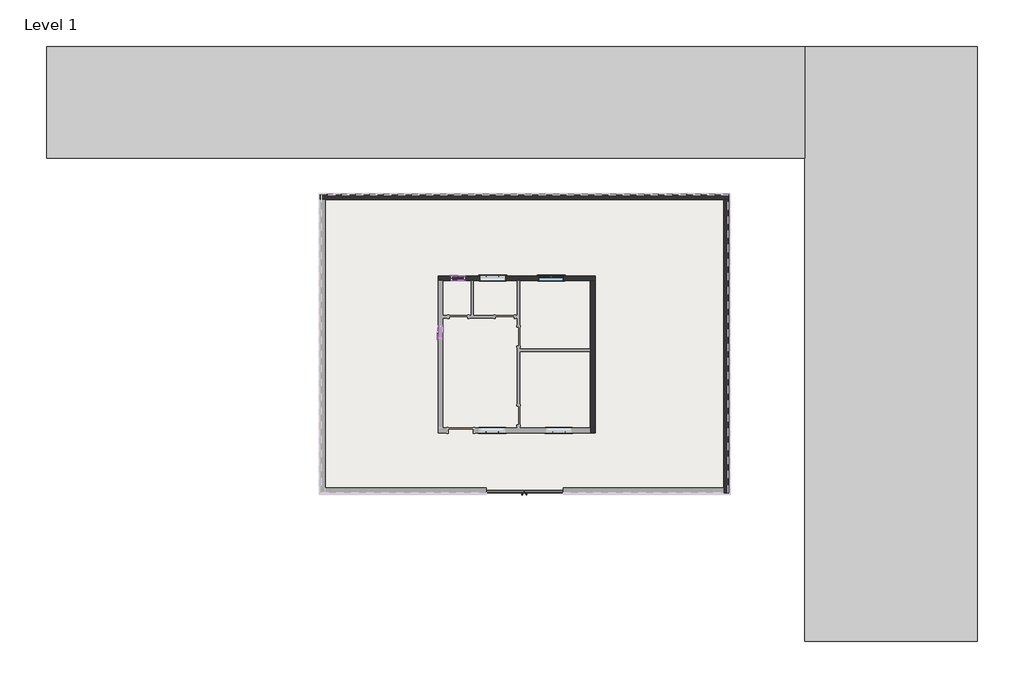
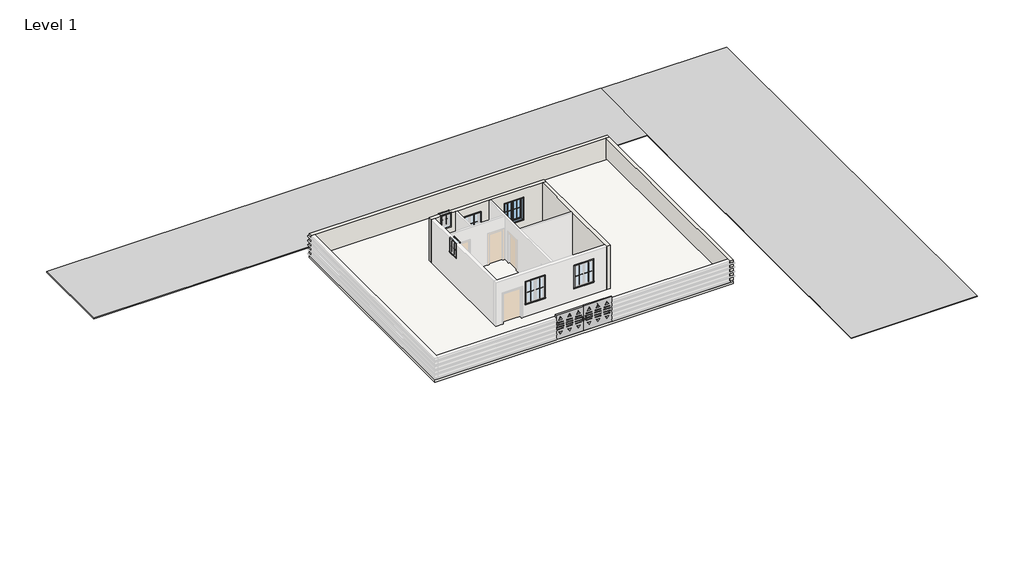
# One storey, part 2 of 2: 26 proxies, 4 walls, 1 slab, 1 window.
"""IFC4 building model written with IfcOpenShell, lengths in millimetres."""

from ifc_helpers import new_model, si_unit, frame, origin, place, context, project, spatial, polyline, outline, extrude, faceted_brep, transform, mapped, element, save
from components import generic_models_afecbd1f, generic_models_1_generic_models_1_fe68cf6e, muntin_pattern_2x2_muntin_pattern_2x2_6dad3731, muntin_pattern_2x2_muntin_pattern_2x2_a30a3345, muntin_pattern_2x2_muntin_pattern_2x2_53152e2c, muntin_pattern_2x2_muntin_pattern_2x2_e8f3e573, trim_window_exterior_flat_with_sill_92b9b949, trim_window_exterior_flat_with_sill_a665a915, trim_window_interior_flat_picture_frame_3bb882cf, trim_window_interior_flat_picture_frame_d485c387, window_8377141f

model = new_model("IFC4")

# Units and contexts
model_context = context("Model", 3, world=origin())
ifc_project = project(units=[si_unit("LENGTHUNIT", "METRE", prefix="MILLI")], contexts=[model_context])

# Site, building, storey
site = spatial("IfcSite", under=ifc_project)
building = spatial("IfcBuilding", under=site)
storey = spatial("IfcBuildingStorey", under=building, Name="Level 1", Elevation=0.0)

# Proxies
placement = place(None, origin())
generic_models_shape = generic_models_afecbd1f(model_context)
element("IfcBuildingElementProxy", 1, Name="Generic Models", at=placement, inside=storey, context=model_context, shape_type="MappedRepresentation", body=[
    mapped(generic_models_shape, transform((4902.2, 3557.455505, 0.0), x_axis=(1.0, 0.0, 0.0), y_axis=(0.0, 1.0, 0.0), z_axis=(0.0, 0.0, 1.0))),
])
generic_models_1_generic_models_1_shape = generic_models_1_generic_models_1_fe68cf6e(model_context)
element("IfcBuildingElementProxy", 2, Name="Generic Models 1 : Generic Models 1", ObjectType="Generic Models 1 : Generic Models 1", at=placement, inside=storey, context=model_context, shape_type="MappedRepresentation", body=[
    mapped(generic_models_1_generic_models_1_shape, transform((0.0, 0.0, 0.0), x_axis=(1.0, 0.0, 0.0), y_axis=(0.0, 1.0, 0.0), z_axis=(0.0, 0.0, 1.0))),
])
muntin_pattern_2x2_muntin_pattern_2x2_shape = muntin_pattern_2x2_muntin_pattern_2x2_6dad3731(model_context)
element("IfcBuildingElementProxy", 3, Name="Muntin Pattern_2x2 : Muntin Pattern_2x2", ObjectType="Muntin Pattern_2x2 : Muntin Pattern_2x2", at=placement, inside=storey, context=model_context, shape_type="MappedRepresentation", body=[
    mapped(muntin_pattern_2x2_muntin_pattern_2x2_shape, transform((6199.1875, 13960.475, 984.25), x_axis=(1.0, 0.0, 0.0), y_axis=(0.0, 1.0, 0.0), z_axis=(0.0, 0.0, 1.0))),
])
element("IfcBuildingElementProxy", 4, Name="Muntin Pattern_2x2 : Muntin Pattern_2x2", ObjectType="Muntin Pattern_2x2 : Muntin Pattern_2x2", at=placement, inside=storey, context=model_context, shape_type="MappedRepresentation", body=[
    mapped(muntin_pattern_2x2_muntin_pattern_2x2_shape, transform((7186.6125, 6359.525, 984.25), x_axis=(-1.0, 0.0, 0.0), y_axis=(0.0, -1.0, 0.0), z_axis=(0.0, 0.0, 1.0))),
])
element("IfcBuildingElementProxy", 5, Name="Muntin Pattern_2x2 : Muntin Pattern_2x2", ObjectType="Muntin Pattern_2x2 : Muntin Pattern_2x2", at=placement, inside=storey, context=model_context, shape_type="MappedRepresentation", body=[
    mapped(muntin_pattern_2x2_muntin_pattern_2x2_shape, transform((3948.1125, 6359.525, 984.25), x_axis=(-1.0, 0.0, 0.0), y_axis=(0.0, -1.0, 0.0), z_axis=(0.0, 0.0, 1.0))),
])
element("IfcBuildingElementProxy", 6, Name="Muntin Pattern_2x2 : Muntin Pattern_2x2", ObjectType="Muntin Pattern_2x2 : Muntin Pattern_2x2", at=placement, inside=storey, context=model_context, shape_type="MappedRepresentation", body=[
    mapped(muntin_pattern_2x2_muntin_pattern_2x2_shape, transform((3360.7375, 13960.475, 984.25), x_axis=(1.0, 0.0, 0.0), y_axis=(0.0, 1.0, 0.0), z_axis=(0.0, 0.0, 1.0))),
])
muntin_pattern_2x2_muntin_pattern_2x2_2_shape = muntin_pattern_2x2_muntin_pattern_2x2_a30a3345(model_context)
element("IfcBuildingElementProxy", 7, Name="Muntin Pattern_2x2 : Muntin Pattern_2x2", ObjectType="Muntin Pattern_2x2 : Muntin Pattern_2x2", at=placement, inside=storey, context=model_context, shape_type="MappedRepresentation", body=[
    mapped(muntin_pattern_2x2_muntin_pattern_2x2_2_shape, transform((6805.6125, 13960.475, 984.25), x_axis=(-1.0, 0.0, 0.0), y_axis=(0.0, -1.0, 0.0), z_axis=(0.0, 0.0, 1.0))),
])
element("IfcBuildingElementProxy", 8, Name="Muntin Pattern_2x2 : Muntin Pattern_2x2", ObjectType="Muntin Pattern_2x2 : Muntin Pattern_2x2", at=placement, inside=storey, context=model_context, shape_type="MappedRepresentation", body=[
    mapped(muntin_pattern_2x2_muntin_pattern_2x2_2_shape, transform((6580.1875, 6359.525, 984.25), x_axis=(1.0, 0.0, 0.0), y_axis=(0.0, 1.0, 0.0), z_axis=(0.0, 0.0, 1.0))),
])
element("IfcBuildingElementProxy", 9, Name="Muntin Pattern_2x2 : Muntin Pattern_2x2", ObjectType="Muntin Pattern_2x2 : Muntin Pattern_2x2", at=placement, inside=storey, context=model_context, shape_type="MappedRepresentation", body=[
    mapped(muntin_pattern_2x2_muntin_pattern_2x2_2_shape, transform((3341.6875, 6359.525, 984.25), x_axis=(1.0, 0.0, 0.0), y_axis=(0.0, 1.0, 0.0), z_axis=(0.0, 0.0, 1.0))),
])
element("IfcBuildingElementProxy", 10, Name="Muntin Pattern_2x2 : Muntin Pattern_2x2", ObjectType="Muntin Pattern_2x2 : Muntin Pattern_2x2", at=placement, inside=storey, context=model_context, shape_type="MappedRepresentation", body=[
    mapped(muntin_pattern_2x2_muntin_pattern_2x2_2_shape, transform((3967.1625, 13960.475, 984.25), x_axis=(-1.0, 0.0, 0.0), y_axis=(0.0, -1.0, 0.0), z_axis=(0.0, 0.0, 1.0))),
])
muntin_pattern_2x2_muntin_pattern_2x2_3_shape = muntin_pattern_2x2_muntin_pattern_2x2_53152e2c(model_context)
element("IfcBuildingElementProxy", 11, Name="Muntin Pattern_2x2 : Muntin Pattern_2x2", ObjectType="Muntin Pattern_2x2 : Muntin Pattern_2x2", at=placement, inside=storey, context=model_context, shape_type="MappedRepresentation", body=[
    mapped(muntin_pattern_2x2_muntin_pattern_2x2_3_shape, transform((1025.525, 11069.6375, 2203.45), x_axis=(0.0, 1.0, 0.0), y_axis=(-1.0, 0.0, 0.0), z_axis=(0.0, 0.0, 1.0))),
])
element("IfcBuildingElementProxy", 12, Name="Muntin Pattern_2x2 : Muntin Pattern_2x2", ObjectType="Muntin Pattern_2x2 : Muntin Pattern_2x2", at=placement, inside=storey, context=model_context, shape_type="MappedRepresentation", body=[
    mapped(muntin_pattern_2x2_muntin_pattern_2x2_3_shape, transform((1830.3875, 13960.475, 2203.45), x_axis=(1.0, 0.0, 0.0), y_axis=(0.0, 1.0, 0.0), z_axis=(0.0, 0.0, 1.0))),
])
muntin_pattern_2x2_muntin_pattern_2x2_4_shape = muntin_pattern_2x2_muntin_pattern_2x2_e8f3e573(model_context)
element("IfcBuildingElementProxy", 13, Name="Muntin Pattern_2x2 : Muntin Pattern_2x2", ObjectType="Muntin Pattern_2x2 : Muntin Pattern_2x2", at=placement, inside=storey, context=model_context, shape_type="MappedRepresentation", body=[
    mapped(muntin_pattern_2x2_muntin_pattern_2x2_4_shape, transform((1025.525, 11371.2625, 2203.45), x_axis=(0.0, -1.0, 0.0), y_axis=(1.0, 0.0, 0.0), z_axis=(0.0, 0.0, 1.0))),
])
element("IfcBuildingElementProxy", 14, Name="Muntin Pattern_2x2 : Muntin Pattern_2x2", ObjectType="Muntin Pattern_2x2 : Muntin Pattern_2x2", at=placement, inside=storey, context=model_context, shape_type="MappedRepresentation", body=[
    mapped(muntin_pattern_2x2_muntin_pattern_2x2_4_shape, transform((2132.0125, 13960.475, 2203.45), x_axis=(-1.0, 0.0, 0.0), y_axis=(0.0, -1.0, 0.0), z_axis=(0.0, 0.0, 1.0))),
])
trim_window_exterior_flat_with_sill_shape = trim_window_exterior_flat_with_sill_92b9b949(model_context)
element("IfcBuildingElementProxy", 15, Name="Trim-Window-Exterior-Flat : with Sill", ObjectType="Trim-Window-Exterior-Flat : with Sill", at=placement, inside=storey, context=model_context, shape_type="MappedRepresentation", body=[
    mapped(trim_window_exterior_flat_with_sill_shape, transform((6502.4, 13970.0, 2438.4), x_axis=(-1.0, 0.0, 0.0), y_axis=(0.0, 0.0, 1.0), z_axis=(0.0, 1.0, 0.0))),
])
element("IfcBuildingElementProxy", 16, Name="Trim-Window-Exterior-Flat : with Sill", ObjectType="Trim-Window-Exterior-Flat : with Sill", at=placement, inside=storey, context=model_context, shape_type="MappedRepresentation", body=[
    mapped(trim_window_exterior_flat_with_sill_shape, transform((6883.4, 6350.0, 2438.4), x_axis=(1.0, 0.0, 0.0), y_axis=(0.0, 0.0, 1.0), z_axis=(0.0, -1.0, 0.0))),
])
element("IfcBuildingElementProxy", 17, Name="Trim-Window-Exterior-Flat : with Sill", ObjectType="Trim-Window-Exterior-Flat : with Sill", at=placement, inside=storey, context=model_context, shape_type="MappedRepresentation", body=[
    mapped(trim_window_exterior_flat_with_sill_shape, transform((3644.9, 6350.0, 2438.4), x_axis=(1.0, 0.0, 0.0), y_axis=(0.0, 0.0, 1.0), z_axis=(0.0, -1.0, 0.0))),
])
element("IfcBuildingElementProxy", 18, Name="Trim-Window-Exterior-Flat : with Sill", ObjectType="Trim-Window-Exterior-Flat : with Sill", at=placement, inside=storey, context=model_context, shape_type="MappedRepresentation", body=[
    mapped(trim_window_exterior_flat_with_sill_shape, transform((3663.95, 13970.0, 2438.4), x_axis=(-1.0, 0.0, 0.0), y_axis=(0.0, 0.0, 1.0), z_axis=(0.0, 1.0, 0.0))),
])
trim_window_exterior_flat_with_sill_2_shape = trim_window_exterior_flat_with_sill_a665a915(model_context)
element("IfcBuildingElementProxy", 19, Name="Trim-Window-Exterior-Flat : with Sill", ObjectType="Trim-Window-Exterior-Flat : with Sill", at=placement, inside=storey, context=model_context, shape_type="MappedRepresentation", body=[
    mapped(trim_window_exterior_flat_with_sill_2_shape, transform((1016.0, 11220.45, 3048.0), x_axis=(0.0, -1.0, 0.0), y_axis=(0.0, 0.0, 1.0), z_axis=(-1.0, 0.0, 0.0))),
])
element("IfcBuildingElementProxy", 20, Name="Trim-Window-Exterior-Flat : with Sill", ObjectType="Trim-Window-Exterior-Flat : with Sill", at=placement, inside=storey, context=model_context, shape_type="MappedRepresentation", body=[
    mapped(trim_window_exterior_flat_with_sill_2_shape, transform((1981.2, 13970.0, 3048.0), x_axis=(-1.0, 0.0, 0.0), y_axis=(0.0, 0.0, 1.0), z_axis=(0.0, 1.0, 0.0))),
])
trim_window_interior_flat_picture_frame_shape = trim_window_interior_flat_picture_frame_3bb882cf(model_context)
element("IfcBuildingElementProxy", 21, Name="Trim-Window-Interior-Flat : Picture Frame", ObjectType="Trim-Window-Interior-Flat : Picture Frame", at=placement, inside=storey, context=model_context, shape_type="MappedRepresentation", body=[
    mapped(trim_window_interior_flat_picture_frame_shape, transform((6502.4, 13741.4, 2438.4), x_axis=(1.0, 0.0, 0.0), y_axis=(0.0, 0.0, 1.0), z_axis=(0.0, -1.0, 0.0))),
])
element("IfcBuildingElementProxy", 22, Name="Trim-Window-Interior-Flat : Picture Frame", ObjectType="Trim-Window-Interior-Flat : Picture Frame", at=placement, inside=storey, context=model_context, shape_type="MappedRepresentation", body=[
    mapped(trim_window_interior_flat_picture_frame_shape, transform((6883.4, 6578.6, 2438.4), x_axis=(-1.0, 0.0, 0.0), y_axis=(0.0, 0.0, 1.0), z_axis=(0.0, 1.0, 0.0))),
])
element("IfcBuildingElementProxy", 23, Name="Trim-Window-Interior-Flat : Picture Frame", ObjectType="Trim-Window-Interior-Flat : Picture Frame", at=placement, inside=storey, context=model_context, shape_type="MappedRepresentation", body=[
    mapped(trim_window_interior_flat_picture_frame_shape, transform((3644.9, 6578.6, 2438.4), x_axis=(-1.0, 0.0, 0.0), y_axis=(0.0, 0.0, 1.0), z_axis=(0.0, 1.0, 0.0))),
])
element("IfcBuildingElementProxy", 24, Name="Trim-Window-Interior-Flat : Picture Frame", ObjectType="Trim-Window-Interior-Flat : Picture Frame", at=placement, inside=storey, context=model_context, shape_type="MappedRepresentation", body=[
    mapped(trim_window_interior_flat_picture_frame_shape, transform((3663.95, 13741.4, 2438.4), x_axis=(1.0, 0.0, 0.0), y_axis=(0.0, 0.0, 1.0), z_axis=(0.0, -1.0, 0.0))),
])
trim_window_interior_flat_picture_frame_2_shape = trim_window_interior_flat_picture_frame_d485c387(model_context)
element("IfcBuildingElementProxy", 25, Name="Trim-Window-Interior-Flat : Picture Frame", ObjectType="Trim-Window-Interior-Flat : Picture Frame", at=placement, inside=storey, context=model_context, shape_type="MappedRepresentation", body=[
    mapped(trim_window_interior_flat_picture_frame_2_shape, transform((1244.6, 11220.45, 3048.0), x_axis=(0.0, 1.0, 0.0), y_axis=(0.0, 0.0, 1.0), z_axis=(1.0, 0.0, 0.0))),
])
element("IfcBuildingElementProxy", 26, Name="Trim-Window-Interior-Flat : Picture Frame", ObjectType="Trim-Window-Interior-Flat : Picture Frame", at=placement, inside=storey, context=model_context, shape_type="MappedRepresentation", body=[
    mapped(trim_window_interior_flat_picture_frame_2_shape, transform((1981.2, 13741.4, 3048.0), x_axis=(1.0, 0.0, 0.0), y_axis=(0.0, 0.0, 1.0), z_axis=(0.0, -1.0, 0.0))),
])

# Slab
element("IfcSlab", 27, ObjectType="Generic - 12\"", at=placement, inside=storey, context=model_context, shape_type="SweptSolid", body=[
    extrude(outline(polyline([(15121.7510144, 17908.455505), (15121.7510144, 3430.455505), (-4690.2489856, 3430.455505), (-4690.2489856, 17908.455505), (15121.7510144, 17908.455505)])), frame((0.0, 0.0, -152.4), z_axis=(0.0, 0.0, 1.0), x_axis=(1.0, 0.0, 0.0)), (0.0, 0.0, 1.0), 152.4),
])

# Walls
element("IfcWall", 28, ObjectType="Generic - 8\"", at=placement, inside=storey, context=model_context, shape_type="Brep", body=[
    faceted_brep([(1016.0, 13741.4, 0.0), (1244.6, 13741.4, 0.0), (2616.2, 13741.4, 0.0), (2730.5, 13741.4, 0.0), (4864.1, 13741.4, 0.0), (4978.4, 13741.4, 0.0), (8407.4, 13741.4, 0.0), (8636.0, 13741.4, 0.0), (8636.0, 13741.4, 3048.0), (8407.4, 13741.4, 3048.0), (4978.4, 13741.4, 3048.0), (4864.1, 13741.4, 3048.0), (2730.5, 13741.4, 3048.0), (2616.2, 13741.4, 3048.0), (2286.0, 13741.4, 3048.0), (2286.0, 13741.4, 2133.6), (1676.4, 13741.4, 2133.6), (1676.4, 13741.4, 3048.0), (1244.6, 13741.4, 3048.0), (1016.0, 13741.4, 3048.0), (7112.0, 13741.4, 2438.4), (7112.0, 13741.4, 914.4), (5892.8, 13741.4, 914.4), (5892.8, 13741.4, 2438.4), (4273.55, 13741.4, 2438.4), (4273.55, 13741.4, 914.4), (3054.35, 13741.4, 914.4), (3054.35, 13741.4, 2438.4), (8636.0, 13970.0, 0.0), (1016.0, 13970.0, 0.0), (1016.0, 13970.0, 3048.0), (1676.4, 13970.0, 3048.0), (1676.4, 13970.0, 2133.6), (2286.0, 13970.0, 2133.6), (2286.0, 13970.0, 3048.0), (8636.0, 13970.0, 3048.0), (7112.0, 13970.0, 914.4), (7112.0, 13970.0, 2438.4), (5892.8, 13970.0, 2438.4), (5892.8, 13970.0, 914.4), (4273.55, 13970.0, 914.4), (4273.55, 13970.0, 2438.4), (3054.35, 13970.0, 2438.4), (3054.35, 13970.0, 914.4)], [[[0, 1, 2, 3, 4, 5, 6, 7, 8, 9, 10, 11, 12, 13, 14, 15, 16, 17, 18, 19], [20, 21, 22, 23], [24, 25, 26, 27]], [[28, 29, 30, 31, 32, 33, 34, 35], [36, 37, 38, 39], [40, 41, 42, 43]], [[7, 6, 5, 4, 3, 2, 1, 0, 29, 28]], [[8, 7, 28, 35]], [[0, 19, 30, 29]], [[21, 20, 37, 36]], [[22, 21, 36, 39]], [[23, 22, 39, 38]], [[20, 23, 38, 37]], [[25, 24, 41, 40]], [[26, 25, 40, 43]], [[27, 26, 43, 42]], [[24, 27, 42, 41]], [[8, 35, 34, 14, 13, 12, 11, 10, 9]], [[30, 19, 18, 17, 31]], [[33, 15, 14, 34]], [[15, 33, 32, 16]], [[16, 32, 31, 17]]]),
])
element("IfcWall", 29, ObjectType="Generic - 8\"", at=placement, inside=storey, context=model_context, shape_type="Brep", body=[
    faceted_brep([(8407.4, 13741.4, 0.0), (8407.4, 10414.0, 0.0), (8407.4, 10299.7, 0.0), (8407.4, 6578.6, 0.0), (8407.4, 6350.0, 0.0), (8407.4, 6350.0, 3048.0), (8407.4, 6578.6, 3048.0), (8407.4, 10299.7, 3048.0), (8407.4, 10414.0, 3048.0), (8407.4, 13741.4, 3048.0), (8636.0, 13741.4, 0.0), (8636.0, 13741.4, 3048.0), (8636.0, 6350.0, 3048.0), (8636.0, 6350.0, 0.0)], [[[0, 1, 2, 3, 4, 5, 6, 7, 8, 9]], [[10, 11, 12, 13]], [[4, 3, 2, 1, 0, 10, 13]], [[0, 9, 11, 10]], [[5, 4, 13, 12]], [[9, 8, 7, 6, 5, 12, 11]]]),
])
element("IfcWall", 30, ObjectType="Generic - 8\"", at=placement, inside=storey, context=model_context, shape_type="Brep", body=[
    faceted_brep([(-4690.2489856, 17679.855505, 0.0), (-4461.6489856, 17679.855505, 0.0), (15121.7510144, 17679.855505, 0.0), (15121.7510144, 17679.855505, 118.9234025), (15121.7510144, 17679.855505, 381.0), (15096.3510144, 17679.855505, 381.0), (15096.3510144, 17679.855505, 448.7333333), (15121.7510144, 17679.855505, 448.7333333), (15121.7510144, 17679.855505, 685.8), (15096.3510144, 17679.855505, 685.8), (15096.3510144, 17679.855505, 753.5333333), (15121.7510144, 17679.855505, 753.5333333), (15121.7510144, 17679.855505, 990.6), (15096.3510144, 17679.855505, 990.6), (15096.3510144, 17679.855505, 1058.3333333), (15121.7510144, 17679.855505, 1058.3333333), (15121.7510144, 17679.855505, 1295.4), (15096.3510144, 17679.855505, 1295.4), (15096.3510144, 17679.855505, 1363.1333333), (15121.7510144, 17679.855505, 1363.1333333), (15121.7510144, 17679.855505, 1524.0), (14893.1510144, 17679.855505, 1524.0), (-4461.6489856, 17679.855505, 1524.0), (-4690.2489856, 17679.855505, 1524.0), (-4690.2489856, 17679.855505, 1363.1333333), (-4664.8489856, 17679.855505, 1363.1333333), (-4664.8489856, 17679.855505, 1295.4), (-4690.2489856, 17679.855505, 1295.4), (-4690.2489856, 17679.855505, 1058.3333333), (-4664.8489856, 17679.855505, 1058.3333333), (-4664.8489856, 17679.855505, 990.6), (-4690.2489856, 17679.855505, 990.6), (-4690.2489856, 17679.855505, 753.5333333), (-4664.8489856, 17679.855505, 753.5333333), (-4664.8489856, 17679.855505, 685.8), (-4690.2489856, 17679.855505, 685.8), (-4690.2489856, 17679.855505, 448.7333333), (-4664.8489856, 17679.855505, 448.7333333), (-4664.8489856, 17679.855505, 381.0), (-4690.2489856, 17679.855505, 381.0), (-4690.2489856, 17679.855505, 143.9333333), (-4664.8489856, 17679.855505, 143.9333333), (-4664.8489856, 17679.855505, 76.2), (-4690.2489856, 17679.855505, 76.2), (15121.7510144, 17908.455505, 0.0), (-4690.2489856, 17908.455505, 0.0), (-4690.2489856, 17908.455505, 76.2), (15121.7510144, 17908.455505, 76.2), (-4690.2489856, 17908.455505, 1524.0), (15121.7510144, 17908.455505, 1524.0), (15121.7510144, 17908.455505, 1363.1333333), (-4690.2489856, 17908.455505, 1363.1333333), (15121.7510144, 17908.455505, 143.9333333), (-4690.2489856, 17908.455505, 143.9333333), (-4690.2489856, 17908.455505, 381.0), (15121.7510144, 17908.455505, 381.0), (15121.7510144, 17908.455505, 448.7333333), (-4690.2489856, 17908.455505, 448.7333333), (-4690.2489856, 17908.455505, 685.8), (15121.7510144, 17908.455505, 685.8), (15121.7510144, 17908.455505, 753.5333333), (-4690.2489856, 17908.455505, 753.5333333), (-4690.2489856, 17908.455505, 990.6), (15121.7510144, 17908.455505, 990.6), (15121.7510144, 17908.455505, 1058.3333333), (-4690.2489856, 17908.455505, 1058.3333333), (-4690.2489856, 17908.455505, 1295.4), (15121.7510144, 17908.455505, 1295.4), (15121.7510144, 17883.055505, 76.2), (15121.7510144, 17883.055505, 143.9333333), (-4664.8489856, 17883.055505, 143.9333333), (-4664.8489856, 17883.055505, 76.2), (15096.3510144, 17883.055505, 448.7333333), (-4664.8489856, 17883.055505, 448.7333333), (-4664.8489856, 17883.055505, 381.0), (15096.3510144, 17883.055505, 381.0), (15096.3510144, 17883.055505, 753.5333333), (-4664.8489856, 17883.055505, 753.5333333), (-4664.8489856, 17883.055505, 685.8), (15096.3510144, 17883.055505, 685.8), (15096.3510144, 17883.055505, 1058.3333333), (-4664.8489856, 17883.055505, 1058.3333333), (-4664.8489856, 17883.055505, 990.6), (15096.3510144, 17883.055505, 990.6), (15096.3510144, 17883.055505, 1363.1333333), (-4664.8489856, 17883.055505, 1363.1333333), (-4664.8489856, 17883.055505, 1295.4), (15096.3510144, 17883.055505, 1295.4)], [[[0, 1, 2, 3, 4, 5, 6, 7, 8, 9, 10, 11, 12, 13, 14, 15, 16, 17, 18, 19, 20, 21, 22, 23, 24, 25, 26, 27, 28, 29, 30, 31, 32, 33, 34, 35, 36, 37, 38, 39, 40, 41, 42, 43]], [[44, 45, 46, 47]], [[48, 49, 50, 51]], [[52, 53, 54, 55]], [[56, 57, 58, 59]], [[60, 61, 62, 63]], [[64, 65, 66, 67]], [[2, 1, 0, 45, 44]], [[23, 22, 21, 20, 49, 48]], [[2, 44, 47, 68, 69, 52, 55, 4, 3]], [[49, 20, 19, 50]], [[7, 56, 59, 8]], [[11, 60, 63, 12]], [[15, 64, 67, 16]], [[23, 48, 51, 24]], [[45, 0, 43, 46]], [[53, 40, 39, 54]], [[57, 36, 35, 58]], [[61, 32, 31, 62]], [[65, 28, 27, 66]], [[69, 70, 41, 40, 53, 52]], [[71, 68, 47, 46, 43, 42]], [[70, 71, 42, 41]], [[70, 69, 68, 71]], [[72, 73, 37, 36, 57, 56, 7, 6]], [[74, 75, 5, 4, 55, 54, 39, 38]], [[73, 74, 38, 37]], [[73, 72, 75, 74]], [[75, 72, 6, 5]], [[76, 77, 33, 32, 61, 60, 11, 10]], [[78, 79, 9, 8, 59, 58, 35, 34]], [[77, 78, 34, 33]], [[77, 76, 79, 78]], [[79, 76, 10, 9]], [[80, 81, 29, 28, 65, 64, 15, 14]], [[82, 83, 13, 12, 63, 62, 31, 30]], [[81, 82, 30, 29]], [[81, 80, 83, 82]], [[83, 80, 14, 13]], [[84, 85, 25, 24, 51, 50, 19, 18]], [[86, 87, 17, 16, 67, 66, 27, 26]], [[85, 86, 26, 25]], [[85, 84, 87, 86]], [[87, 84, 18, 17]]]),
])
element("IfcWall", 31, ObjectType="Generic - 8\"", at=placement, inside=storey, context=model_context, shape_type="Brep", body=[
    faceted_brep([(14893.1510144, 17679.855505, 118.9234025), (14893.1510144, 3430.455505, 118.9234025), (14893.1510144, 3430.455505, 143.9333333), (14893.1510144, 3430.455505, 381.0), (14893.1510144, 3455.855505, 381.0), (14893.1510144, 3455.855505, 448.7333333), (14893.1510144, 3430.455505, 448.7333333), (14893.1510144, 3430.455505, 685.8), (14893.1510144, 3455.855505, 685.8), (14893.1510144, 3455.855505, 753.5333333), (14893.1510144, 3430.455505, 753.5333333), (14893.1510144, 3430.455505, 990.6), (14893.1510144, 3455.855505, 990.6), (14893.1510144, 3455.855505, 1058.3333333), (14893.1510144, 3430.455505, 1058.3333333), (14893.1510144, 3430.455505, 1295.4), (14893.1510144, 3455.855505, 1295.4), (14893.1510144, 3455.855505, 1363.1333333), (14893.1510144, 3430.455505, 1363.1333333), (14893.1510144, 3430.455505, 1524.0), (14893.1510144, 3659.055505, 1524.0), (14893.1510144, 17679.855505, 1524.0), (15121.7510144, 3430.455505, 118.9234025), (15121.7510144, 17679.855505, 118.9234025), (15121.7510144, 17679.855505, 381.0), (15121.7510144, 3430.455505, 381.0), (15121.7510144, 17679.855505, 1524.0), (15121.7510144, 3430.455505, 1524.0), (15121.7510144, 3430.455505, 1363.1333333), (15121.7510144, 17679.855505, 1363.1333333), (15121.7510144, 3430.455505, 448.7333333), (15121.7510144, 17679.855505, 448.7333333), (15121.7510144, 17679.855505, 685.8), (15121.7510144, 3430.455505, 685.8), (15121.7510144, 3430.455505, 753.5333333), (15121.7510144, 17679.855505, 753.5333333), (15121.7510144, 17679.855505, 990.6), (15121.7510144, 3430.455505, 990.6), (15121.7510144, 3430.455505, 1058.3333333), (15121.7510144, 17679.855505, 1058.3333333), (15121.7510144, 17679.855505, 1295.4), (15121.7510144, 3430.455505, 1295.4), (15096.3510144, 17679.855505, 1363.1333333), (15096.3510144, 17679.855505, 1295.4), (15096.3510144, 17679.855505, 1058.3333333), (15096.3510144, 17679.855505, 990.6), (15096.3510144, 17679.855505, 753.5333333), (15096.3510144, 17679.855505, 685.8), (15096.3510144, 17679.855505, 448.7333333), (15096.3510144, 17679.855505, 381.0), (15096.3510144, 3455.855505, 448.7333333), (15096.3510144, 3455.855505, 381.0), (15096.3510144, 3455.855505, 753.5333333), (15096.3510144, 3455.855505, 685.8), (15096.3510144, 3455.855505, 1058.3333333), (15096.3510144, 3455.855505, 990.6), (15096.3510144, 3455.855505, 1363.1333333), (15096.3510144, 3455.855505, 1295.4)], [[[0, 1, 2, 3, 4, 5, 6, 7, 8, 9, 10, 11, 12, 13, 14, 15, 16, 17, 18, 19, 20, 21]], [[22, 23, 24, 25]], [[26, 27, 28, 29]], [[30, 31, 32, 33]], [[34, 35, 36, 37]], [[38, 39, 40, 41]], [[1, 0, 23, 22]], [[21, 20, 19, 27, 26]], [[0, 21, 26, 29, 42, 43, 40, 39, 44, 45, 36, 35, 46, 47, 32, 31, 48, 49, 24, 23]], [[1, 22, 25, 3, 2]], [[27, 19, 18, 28]], [[6, 30, 33, 7]], [[10, 34, 37, 11]], [[14, 38, 41, 15]], [[5, 50, 48, 31, 30, 6]], [[49, 51, 4, 3, 25, 24]], [[50, 51, 49, 48]], [[51, 50, 5, 4]], [[9, 52, 46, 35, 34, 10]], [[47, 53, 8, 7, 33, 32]], [[52, 53, 47, 46]], [[53, 52, 9, 8]], [[13, 54, 44, 39, 38, 14]], [[45, 55, 12, 11, 37, 36]], [[54, 55, 45, 44]], [[55, 54, 13, 12]], [[17, 56, 42, 29, 28, 18]], [[43, 57, 16, 15, 41, 40]], [[56, 57, 43, 42]], [[57, 56, 17, 16]]]),
])

# Window
window_shape = window_8377141f(model_context)
element("IfcWindow", 32, ObjectType="Window-Casement-Double : 48\" x 60\"", at=placement, inside=storey, context=model_context, shape_type="MappedRepresentation", body=[
    mapped(window_shape, transform((6502.4, 13855.7, 0.0), x_axis=(1.0, 0.0, 0.0), y_axis=(0.0, 1.0, 0.0), z_axis=(0.0, 0.0, 1.0))),
])

save(model, "model.ifc")

# Revit data of these elements
# Type
#   Default Elevation = 0
# Type "Muntin Pattern_2x2 : Muntin Pattern_2x2"
#   Width [instance default] = 4' - 0"
#   Thickness = 0' - 0 1/2"
#   Height [instance default] = 4' - 0"
#   Distance = 0' - 0 3/4"
#   Interior Material [instance default] = none
#   Exterior Material [instance default] = none
#   Default Elevation = 0
# Type "Trim-Window-Exterior-Flat : with Sill"
#   Trim Width = 0' - 2 1/4"
#   Trim Thickness_Picture Frame = 0' - 1 1/4"
#   Trim Thickness_with Sill = 0' - 0 3/4"
#   Sill Thickness = 0' - 1 1/4"
#   Opening Width [instance default] = 2' - 0"
#   Opening Height [instance default] = 3' - 0"
#   Default Elevation = 4' - 0"
#   Sill = yes
#   Picture Frame = no
#   Trim Material [instance default] = none
# Type "Trim-Window-Interior-Flat : Picture Frame"
#   Trim Thickness_Picture Frame = 0' - 1 1/4"
#   Trim Width = 0' - 2 1/4"
#   Trim Thickness_with Sill = 0' - 0 3/4"
#   Sill Thickness = 0' - 1 1/4"
#   Opening Width [instance default] = 2' - 0"
#   Opening Height [instance default] = 3' - 0"
#   Default Elevation = 4' - 0"
#   Sill = no
#   Picture Frame = yes
#   Trim Material [instance default] = none
# Type "Generic - 12\""
#   Assembly Code = "B1010"
#   Function = 0
#   Layers, outside or top first: 0' - 6" no material (function 1)
# Type "Generic - 8\""
#   Assembly Code = "B2010"
#   Layers, outside or top first: 0' - 9" "Parking Stripe" (function 1)
# Type "Window-Casement-Double : 48\" x 60\""
#   Type Mark = "17"
#   Fire Rating = "0.5h"
#   Assembly Code = "B2020100"
#   Analytic Construction = "Double glazing - domestic"
#   Frame Extension [instance default] = 0' - 0 1/4"
#   Window Inset [instance default] = 0' - 0"
#   Wall Thickness [instance default] = 0' - 6"
#   Interior Wall Closure [instance default] = 0' - 2 1/4"
#   Half Width = 2' - 0"
#   Visual Light Transmittance = 0.81
#   Thermal Resistance (R) = 1.8146 (h·ft²·°F)/BTU
#   Solar Heat Gain Coefficient = 0.76
#   Rough Width = 4' - 0 1/2"
#   Rough Height = 5' - 0 1/2"
#   Height = 5' - 0"
#   Heat Transfer Coefficient (U) = 0.5511 BTU/(h·ft²·°F)
#   Exterior Wall Closure [instance default] = 0' - 1 1/4"
#   Extension Jamb [instance default] = 0' - 2 1/4"
#   Default Sill Height = 3' - 0"
#   Width = 4' - 0"
#   Define Thermal Properties by = 0
#   Muntin Visibility = yes
#   Interior Trim Visibility [instance default] = yes
#   Exterior Trim Visibility [instance default] = yes
#   Extension Jamb Visibility [instance default] = yes
#   Interior Trim Material = Wood - Stained
#   Muntin Pattern = Muntin Pattern_2x2 : Muntin Pattern_2x2
#   Interior Trim = Trim-Window-Interior-Flat : Picture Frame
#   Interior Frame Material = Wood - Stained
#   Glass Panel Material = Glass
#   Exterior Trim Material = Clad - White
#   Exterior Trim = Trim-Window-Exterior-Flat : with Sill
#   Exterior Frame Material = Clad - White
#   Wall Closure = (empty or 0)
# Element 1 (IfcBuildingElementProxy)
#   Phase Created = New Construction
#   Materials on its faces: "GATE"
# Element 2 (IfcBuildingElementProxy, "Generic Models 1 : Generic Models 1")
#   Phase Created = New Construction
# Elements 3, 4, 5, 6, 7, 8, 9, 10 (IfcBuildingElementProxy, "Muntin Pattern_2x2 : Muntin Pattern_2x2")
#   Width = 1' - 6 5/8"
#   Height = 4' - 6 1/2"
#   Interior Material = Wood - Stained
#   Exterior Material = Clad - White
#   Phase Created = New Construction
#   Materials on its faces: "Clad - White", "Wood - Stained"
# Elements 11, 12, 13, 14 (IfcBuildingElementProxy, "Muntin Pattern_2x2 : Muntin Pattern_2x2")
#   Width = 0' - 6 5/8"
#   Height = 2' - 6 1/2"
#   Interior Material = Wood - Stained
#   Exterior Material = Clad - White
#   Phase Created = New Construction
#   Materials on its faces: "Clad - White", "Wood - Stained"
# Elements 15, 16, 17, 18 (IfcBuildingElementProxy, "Trim-Window-Exterior-Flat : with Sill")
#   Opening Width = 4' - 0"
#   Opening Height = 5' - 0"
#   Trim Material = Clad - White
#   Phase Created = New Construction
#   Materials on its faces: "Clad - White"
# Elements 19, 20 (IfcBuildingElementProxy, "Trim-Window-Exterior-Flat : with Sill")
#   Opening Width = 2' - 0"
#   Opening Height = 3' - 0"
#   Trim Material = Clad - White
#   Phase Created = New Construction
#   Materials on its faces: "Clad - White"
# Elements 21, 22, 23, 24 (IfcBuildingElementProxy, "Trim-Window-Interior-Flat : Picture Frame")
#   Opening Width = 4' - 0"
#   Opening Height = 5' - 0"
#   Trim Material = Wood - Stained
#   Phase Created = New Construction
#   Materials on its faces: "Wood - Stained"
# Elements 25, 26 (IfcBuildingElementProxy, "Trim-Window-Interior-Flat : Picture Frame")
#   Opening Width = 2' - 0"
#   Opening Height = 3' - 0"
#   Trim Material = Wood - Stained
#   Phase Created = New Construction
#   Materials on its faces: "Wood - Stained"
# Element 27 (IfcSlab, "Generic - 12\"")
#   Height Offset From Level = 0' - 0"
#   Phase Created = New Construction
#   Materials on its faces: "Plywood, Sheathing", "Default Floor", "Door - Panel"
# Elements 28, 29 (IfcWall, "Generic - 8\"")
#   Top Offset = 0' - 0"
#   Base Offset = 0' - 0"
#   Unconnected Height = 10' - 0"
#   wall height = 10' - 0"
#   Phase Created = New Construction
#   Base Constraint = Level 1
#   Materials on its faces: "Parking Stripe", "Wood Planks"
# Element 30 (IfcWall, "Generic - 8\"")
#   Top Offset = 0' - 0"
#   Base Offset = 0' - 0"
#   Unconnected Height = 5' - 0"
#   wall height = 5' - 0"
#   Phase Created = New Construction
#   Base Constraint = Level 1
#   Materials on its faces: "Parking Stripe", "Plywood, Sheathing", "Textile - Linen, Smooth"
# Element 31 (IfcWall, "Generic - 8\"")
#   built-in parameter 1001111 = 0' - 4.68202"
#   Top Offset = 0' - 0"
#   Base Offset = 0' - 4.68202"
#   Unconnected Height = 4' - 7.31798"
#   wall height = 4' - 7.31798"
#   Phase Created = New Construction
#   Base Constraint = Level 1
#   Materials on its faces: "Parking Stripe", "Plywood, Sheathing", "Textile - Linen, Smooth"
# Element 32 (IfcWindow, "Window-Casement-Double : 48\" x 60\"")
#   Mark = "1"
#   Window Inset = 0' - 0"
#   Interior Wall Closure = 0' - 2 1/4"
#   Frame Extension = 0' - 0 1/4"
#   Exterior Wall Closure = 0' - 1 1/4"
#   Interior Trim Visibility = yes
#   Exterior Trim Visibility = yes
#   Phase Created = New Construction
#   Materials on its faces: "Wood - Stained", "Glass", "Clad - White"
# Materials
#   "Parking Stripe": class "Paint", colour RGB 250 250 91, transparency 0, Cost = 0
#   "Wood - Stained": class "Wood", colour RGB 224 178 126, transparency 0, Cost = 0
#   "Glass": class "Glass", colour RGB 0 128 192, transparency 0.75, Description = "Soda Lime Glass", Cost = 0
#   "Clad - White": class "Wood", colour RGB 242 242 238, transparency 0, Cost = 0
#   "GATE": class "Generic", colour RGB 120 120 120, transparency 0, Cost = 0
#   "Plywood, Sheathing": class "Wood", colour RGB 212 179 113, transparency 0, Description = "Plywood, sheathing grade", Cost = 0
#   "Default Floor": colour RGB 128 128 128, transparency 0, Cost = 0
#   "Door - Panel": class "Wood", colour RGB 210 159 95, transparency 0, Cost = 0
#   "Wood Planks": class "Wood", colour RGB 193 160 115, transparency 0, Description = "Physical material.", Cost = 0
#   "Textile - Linen, Smooth": colour RGB 249 239 230, transparency 0
